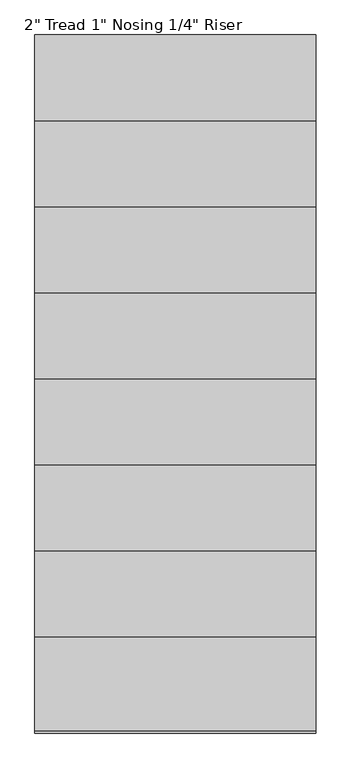
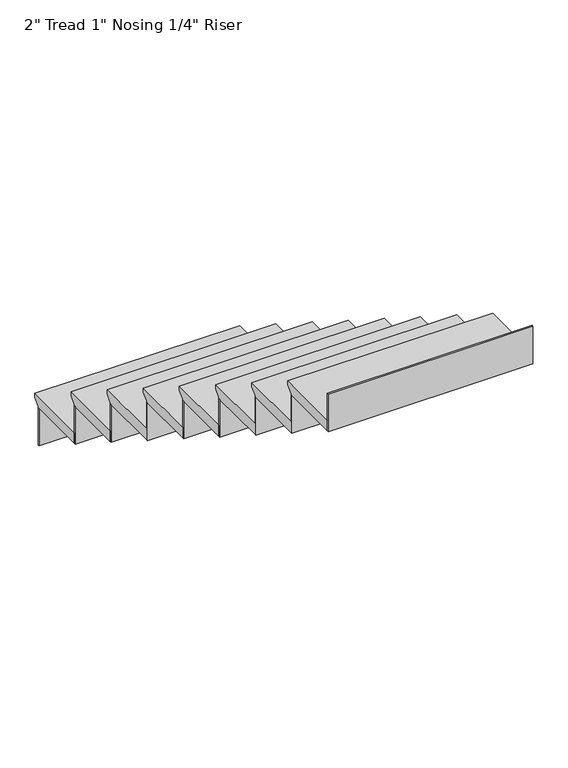
"""IFC4 building model written with IfcOpenShell, lengths in millimetres: stair flight geometry."""

from ifc_helpers import new_model, si_unit, frame, origin, place, context, project, spatial, polyline, outline, extrude, source, transform, mapped, element, save


def stair_flight_9be7654d(model_context):
    return source(origin(), model_context, "Body", "SweptSolid", [
        extrude(outline(polyline([(8107.643496, 5588.0), (8412.443496, 5588.0), (8412.443496, 5568.95), (8387.043496, 5543.55), (8387.043496, 5537.2), (8107.643496, 5537.2), (8107.643496, 5588.0)])), frame((-11538.468339, 0.0, 0.0), z_axis=(1.0, 0.0, 0.0), x_axis=(0.0, 1.0, 0.0)), (0.0, 0.0, 1.0), 914.4),
        extrude(outline(polyline([(-11538.468339, 8380.693496), (-11538.468339, 8387.043496), (-10624.068339, 8387.043496), (-10624.068339, 8380.693496), (-11538.468339, 8380.693496)])), frame((0.0, 0.0, 5359.4), z_axis=(0.0, 0.0, 1.0), x_axis=(1.0, 0.0, 0.0)), (0.0, 0.0, 1.0), 177.8),
        extrude(outline(polyline([(-11538.468339, 8101.293496), (-11538.468339, 8107.643496), (-10624.068339, 8107.643496), (-10624.068339, 8101.293496), (-11538.468339, 8101.293496)])), frame((0.0, 0.0, 5537.2), z_axis=(0.0, 0.0, 1.0), x_axis=(1.0, 0.0, 0.0)), (0.0, 0.0, 1.0), 177.8),
        extrude(outline(polyline([(7828.243496, 5765.8), (8133.043496, 5765.8), (8133.043496, 5746.75), (8107.643496, 5721.35), (8107.643496, 5715.0), (7828.243496, 5715.0), (7828.243496, 5765.8)])), frame((-11538.468339, 0.0, 0.0), z_axis=(1.0, 0.0, 0.0), x_axis=(0.0, 1.0, 0.0)), (0.0, 0.0, 1.0), 914.4),
        extrude(outline(polyline([(-11538.468339, 7821.893496), (-11538.468339, 7828.243496), (-10624.068339, 7828.243496), (-10624.068339, 7821.893496), (-11538.468339, 7821.893496)])), frame((0.0, 0.0, 5715.0), z_axis=(0.0, 0.0, 1.0), x_axis=(1.0, 0.0, 0.0)), (0.0, 0.0, 1.0), 177.8),
        extrude(outline(polyline([(7548.843496, 5943.6), (7853.643496, 5943.6), (7853.643496, 5924.55), (7828.243496, 5899.15), (7828.243496, 5892.8), (7548.843496, 5892.8), (7548.843496, 5943.6)])), frame((-11538.468339, 0.0, 0.0), z_axis=(1.0, 0.0, 0.0), x_axis=(0.0, 1.0, 0.0)), (0.0, 0.0, 1.0), 914.4),
        extrude(outline(polyline([(-11538.468339, 7542.493496), (-11538.468339, 7548.843496), (-10624.068339, 7548.843496), (-10624.068339, 7542.493496), (-11538.468339, 7542.493496)])), frame((0.0, 0.0, 5892.8), z_axis=(0.0, 0.0, 1.0), x_axis=(1.0, 0.0, 0.0)), (0.0, 0.0, 1.0), 177.8),
        extrude(outline(polyline([(7269.443496, 6121.4), (7574.243496, 6121.4), (7574.243496, 6102.35), (7548.843496, 6076.95), (7548.843496, 6070.6), (7269.443496, 6070.6), (7269.443496, 6121.4)])), frame((-11538.468339, 0.0, 0.0), z_axis=(1.0, 0.0, 0.0), x_axis=(0.0, 1.0, 0.0)), (0.0, 0.0, 1.0), 914.4),
        extrude(outline(polyline([(-11538.468339, 7263.093496), (-11538.468339, 7269.443496), (-10624.068339, 7269.443496), (-10624.068339, 7263.093496), (-11538.468339, 7263.093496)])), frame((0.0, 0.0, 6070.6), z_axis=(0.0, 0.0, 1.0), x_axis=(1.0, 0.0, 0.0)), (0.0, 0.0, 1.0), 177.8),
        extrude(outline(polyline([(6990.043496, 6299.2), (7294.843496, 6299.2), (7294.843496, 6280.15), (7269.443496, 6254.75), (7269.443496, 6248.4), (6990.043496, 6248.4), (6990.043496, 6299.2)])), frame((-11538.468339, 0.0, 0.0), z_axis=(1.0, 0.0, 0.0), x_axis=(0.0, 1.0, 0.0)), (0.0, 0.0, 1.0), 914.4),
        extrude(outline(polyline([(-11538.468339, 6983.693496), (-11538.468339, 6990.043496), (-10624.068339, 6990.043496), (-10624.068339, 6983.693496), (-11538.468339, 6983.693496)])), frame((0.0, 0.0, 6248.4), z_axis=(0.0, 0.0, 1.0), x_axis=(1.0, 0.0, 0.0)), (0.0, 0.0, 1.0), 177.8),
        extrude(outline(polyline([(6710.643496, 6477.0), (7015.443496, 6477.0), (7015.443496, 6457.95), (6990.043496, 6432.55), (6990.043496, 6426.2), (6710.643496, 6426.2), (6710.643496, 6477.0)])), frame((-11538.468339, 0.0, 0.0), z_axis=(1.0, 0.0, 0.0), x_axis=(0.0, 1.0, 0.0)), (0.0, 0.0, 1.0), 914.4),
        extrude(outline(polyline([(-11538.468339, 6704.293496), (-11538.468339, 6710.643496), (-10624.068339, 6710.643496), (-10624.068339, 6704.293496), (-11538.468339, 6704.293496)])), frame((0.0, 0.0, 6426.2), z_axis=(0.0, 0.0, 1.0), x_axis=(1.0, 0.0, 0.0)), (0.0, 0.0, 1.0), 177.8),
        extrude(outline(polyline([(6431.243496, 6654.8), (6736.043496, 6654.8), (6736.043496, 6635.75), (6710.643496, 6610.35), (6710.643496, 6604.0), (6431.243496, 6604.0), (6431.243496, 6654.8)])), frame((-11538.468339, 0.0, 0.0), z_axis=(1.0, 0.0, 0.0), x_axis=(0.0, 1.0, 0.0)), (0.0, 0.0, 1.0), 914.4),
        extrude(outline(polyline([(-11538.468339, 6424.893496), (-11538.468339, 6431.243496), (-10624.068339, 6431.243496), (-10624.068339, 6424.893496), (-11538.468339, 6424.893496)])), frame((0.0, 0.0, 6604.0), z_axis=(0.0, 0.0, 1.0), x_axis=(1.0, 0.0, 0.0)), (0.0, 0.0, 1.0), 177.8),
        extrude(outline(polyline([(-11538.468339, 6145.493496), (-11538.468339, 6151.843496), (-10624.068339, 6151.843496), (-10624.068339, 6145.493496), (-11538.468339, 6145.493496)])), frame((0.0, 0.0, 6781.8), z_axis=(0.0, 0.0, 1.0), x_axis=(1.0, 0.0, 0.0)), (0.0, 0.0, 1.0), 177.8),
        extrude(outline(polyline([(6151.843496, 6832.6), (6456.643496, 6832.6), (6456.643496, 6813.55), (6431.243496, 6788.15), (6431.243496, 6781.8), (6151.843496, 6781.8), (6151.843496, 6832.6)])), frame((-11538.468339, 0.0, 0.0), z_axis=(1.0, 0.0, 0.0), x_axis=(0.0, 1.0, 0.0)), (0.0, 0.0, 1.0), 914.4),
    ])


if __name__ == "__main__":
    model = new_model("IFC4")
    model_context = context("Model", 3, world=origin())
    ifc_project = project(units=[si_unit("LENGTHUNIT", "METRE", prefix="MILLI")], contexts=[model_context])
    site = spatial("IfcSite", under=ifc_project)
    building = spatial("IfcBuilding", under=site)
    placement = place(None, origin())
    stair_flight_shape = stair_flight_9be7654d(model_context)
    element("IfcStairFlight", 1, ObjectType="2\" Tread 1\" Nosing 1/4\" Riser", at=placement, inside=building, context=model_context, shape_type="MappedRepresentation", body=[
        mapped(stair_flight_shape, transform((0.0, 0.0, 0.0), x_axis=(1.0, 0.0, 0.0), y_axis=(0.0, 1.0, 0.0), z_axis=(0.0, 0.0, 1.0))),
    ])
    save(model, "model.ifc")
